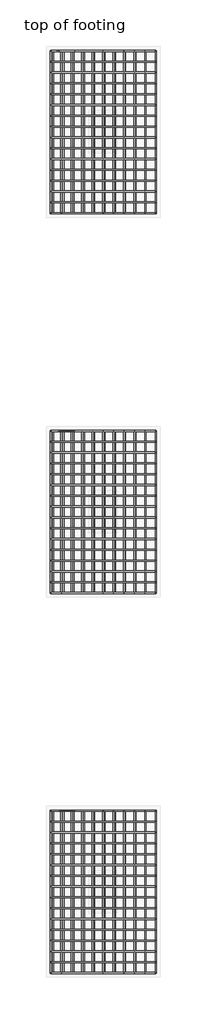
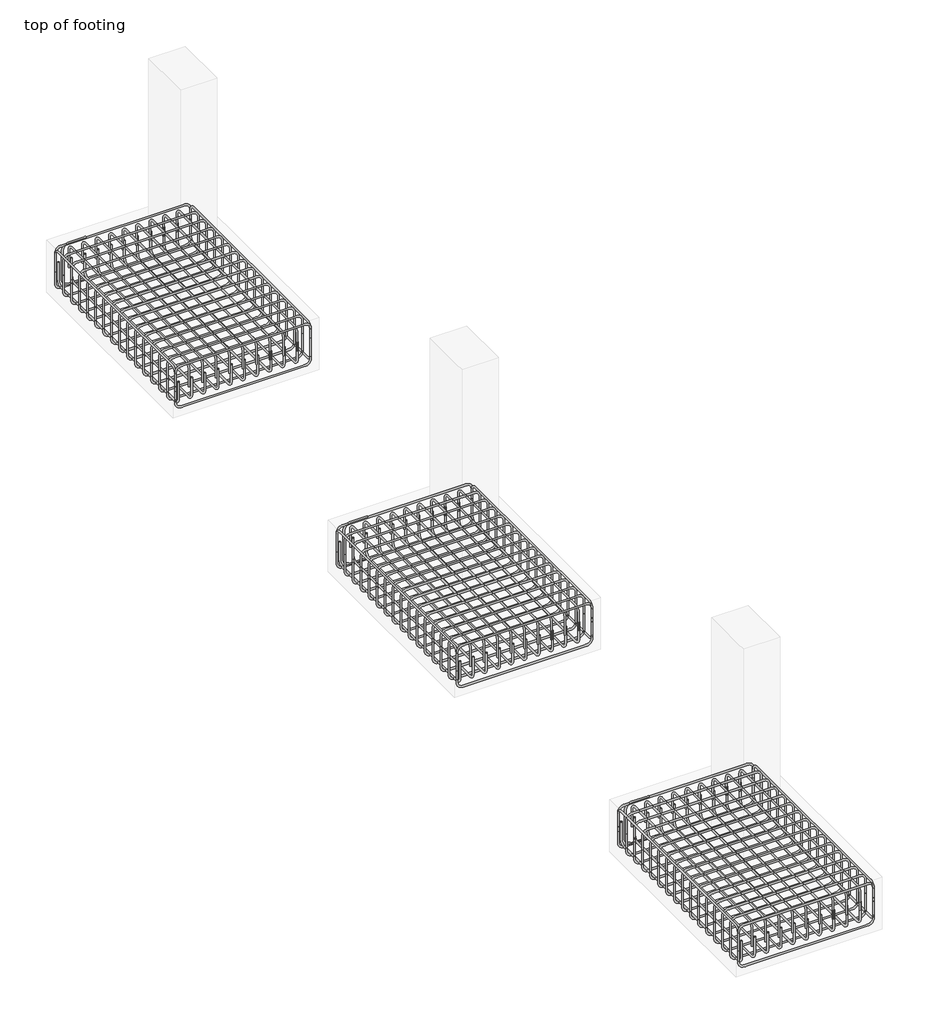
# One storey, part 8 of 8: 15 reinforcing bars.
"""IFC4 building model written with IfcOpenShell, lengths in millimetres."""

from ifc_helpers import new_model, si_unit, point, frame, origin, place, context, project, spatial, polyline, circle_curve, trimmed, segment, composite_curve, source, transform, mapped, element, save
from ifc_brep_helpers import swept_disk

model = new_model("IFC4")

# Units and contexts
model_context = context("Model", 3, world=origin())
ifc_project = project(units=[si_unit("LENGTHUNIT", "METRE", prefix="MILLI")], contexts=[model_context])

# Site, building, storey
site = spatial("IfcSite", under=ifc_project)
building = spatial("IfcBuilding", under=site)
storey = spatial("IfcBuildingStorey", under=building, Name="top of footing", Elevation=-1828.8)

# Reinforcing bars
placement = place(None, origin())
reinforcing_bar_shape = source(origin(), model_context, "Body", "SolidModel", [
    swept_disk(composite_curve([segment(polyline([(3314.5699811, 16682.8075251, -2014.4920065), (3314.5699811, 16682.8075251, -2161.7920065)]), True, "CONTINUOUS"), segment(trimmed(circle_curve(frame((3314.5699811, 16729.1575251, -2161.7920065), z_axis=(1.0, 0.0, 0.0), x_axis=(0.0, -46.349999999998545, 0.0)), 46.35), [point((3314.5699811, 16682.8075251, -2161.7920065))], [point((3314.5699811, 16729.1575251, -2208.1420065))], True, "CARTESIAN"), True, "CONTINUOUS"), segment(polyline([(3314.5699811, 16729.1575251, -2208.1420065), (3314.5699811, 18343.7575251, -2208.1420065)]), True, "CONTINUOUS"), segment(trimmed(circle_curve(frame((3314.5699811, 18343.7575251, -2161.7920065), z_axis=(1.0, 0.0, 0.0), x_axis=(0.0, 0.0, -46.350000000000364)), 46.35), [point((3314.5699811, 18343.7575251, -2208.1420065))], [point((3314.5699811, 18390.1075251, -2161.7920065))], True, "CARTESIAN"), True, "CONTINUOUS"), segment(polyline([(3314.5699811, 18390.1075251, -2161.7920065), (3314.5699811, 18390.1075251, -2014.4920065)]), True, "CONTINUOUS")], self_intersect=False), 6.35),
])
element("IfcReinforcingBar", 1, at=placement, inside=storey, context=model_context, shape_type="MappedRepresentation", body=[
    mapped(reinforcing_bar_shape, transform((0.0, 0.0, 0.0), x_axis=(1.0, 0.0, 0.0), y_axis=(0.0, 1.0, 0.0), z_axis=(0.0, 0.0, 1.0))),
    mapped(reinforcing_bar_shape, transform((-108.3645139, 0.0, 0.0), x_axis=(1.0, 0.0, 0.0), y_axis=(0.0, 1.0, 0.0), z_axis=(0.0, 0.0, 1.0))),
    mapped(reinforcing_bar_shape, transform((-216.7290279, 0.0, 0.0), x_axis=(1.0, 0.0, 0.0), y_axis=(0.0, 1.0, 0.0), z_axis=(0.0, 0.0, 1.0))),
    mapped(reinforcing_bar_shape, transform((-325.0935418, 0.0, 0.0), x_axis=(1.0, 0.0, 0.0), y_axis=(0.0, 1.0, 0.0), z_axis=(0.0, 0.0, 1.0))),
    mapped(reinforcing_bar_shape, transform((-433.4580557, 0.0, 0.0), x_axis=(1.0, 0.0, 0.0), y_axis=(0.0, 1.0, 0.0), z_axis=(0.0, 0.0, 1.0))),
    mapped(reinforcing_bar_shape, transform((-541.8225696, 0.0, 0.0), x_axis=(1.0, 0.0, 0.0), y_axis=(0.0, 1.0, 0.0), z_axis=(0.0, 0.0, 1.0))),
    mapped(reinforcing_bar_shape, transform((-650.1870836, 0.0, 0.0), x_axis=(1.0, 0.0, 0.0), y_axis=(0.0, 1.0, 0.0), z_axis=(0.0, 0.0, 1.0))),
    mapped(reinforcing_bar_shape, transform((-758.5515975, 0.0, 0.0), x_axis=(1.0, 0.0, 0.0), y_axis=(0.0, 1.0, 0.0), z_axis=(0.0, 0.0, 1.0))),
    mapped(reinforcing_bar_shape, transform((-866.9161114, 0.0, 0.0), x_axis=(1.0, 0.0, 0.0), y_axis=(0.0, 1.0, 0.0), z_axis=(0.0, 0.0, 1.0))),
    mapped(reinforcing_bar_shape, transform((-975.2806253, 0.0, 0.0), x_axis=(1.0, 0.0, 0.0), y_axis=(0.0, 1.0, 0.0), z_axis=(0.0, 0.0, 1.0))),
    mapped(reinforcing_bar_shape, transform((-1083.6451393, 0.0, 0.0), x_axis=(1.0, 0.0, 0.0), y_axis=(0.0, 1.0, 0.0), z_axis=(0.0, 0.0, 1.0))),
])
reinforcing_bar_2_shape = source(origin(), model_context, "Body", "SolidModel", [
    swept_disk(composite_curve([segment(polyline([(2207.2699811, 16682.8075251, -2085.8010212), (2207.2699811, 16682.8075251, -1938.5010212)]), True, "CONTINUOUS"), segment(trimmed(circle_curve(frame((2207.2699811, 16729.1575251, -1938.5010212), z_axis=(-1.0, 0.0, 0.0), x_axis=(0.0, -46.349999999998545, 0.0)), 46.35), [point((2207.2699811, 16682.8075251, -1938.5010212))], [point((2207.2699811, 16729.1575251, -1892.1510212))], True, "CARTESIAN"), True, "CONTINUOUS"), segment(polyline([(2207.2699811, 16729.1575251, -1892.1510212), (2207.2699811, 18343.7575251, -1892.1510212)]), True, "CONTINUOUS"), segment(trimmed(circle_curve(frame((2207.2699811, 18343.7575251, -1938.5010212), z_axis=(-1.0, 0.0, 0.0), x_axis=(0.0, 0.0, 46.34999999999991)), 46.35), [point((2207.2699811, 18343.7575251, -1892.1510212))], [point((2207.2699811, 18390.1075251, -1938.5010212))], True, "CARTESIAN"), True, "CONTINUOUS"), segment(polyline([(2207.2699811, 18390.1075251, -1938.5010212), (2207.2699811, 18390.1075251, -2085.8010212)]), True, "CONTINUOUS")], self_intersect=False), 6.35),
])
element("IfcReinforcingBar", 2, at=placement, inside=storey, context=model_context, shape_type="MappedRepresentation", body=[
    mapped(reinforcing_bar_2_shape, transform((0.0, 0.0, 0.0), x_axis=(1.0, 0.0, 0.0), y_axis=(0.0, 1.0, 0.0), z_axis=(0.0, 0.0, 1.0))),
    mapped(reinforcing_bar_2_shape, transform((110.73, 0.0, 0.0), x_axis=(1.0, 0.0, 0.0), y_axis=(0.0, 1.0, 0.0), z_axis=(0.0, 0.0, 1.0))),
    mapped(reinforcing_bar_2_shape, transform((221.46, 0.0, 0.0), x_axis=(1.0, 0.0, 0.0), y_axis=(0.0, 1.0, 0.0), z_axis=(0.0, 0.0, 1.0))),
    mapped(reinforcing_bar_2_shape, transform((332.19, 0.0, 0.0), x_axis=(1.0, 0.0, 0.0), y_axis=(0.0, 1.0, 0.0), z_axis=(0.0, 0.0, 1.0))),
    mapped(reinforcing_bar_2_shape, transform((442.92, 0.0, 0.0), x_axis=(1.0, 0.0, 0.0), y_axis=(0.0, 1.0, 0.0), z_axis=(0.0, 0.0, 1.0))),
    mapped(reinforcing_bar_2_shape, transform((553.65, 0.0, 0.0), x_axis=(1.0, 0.0, 0.0), y_axis=(0.0, 1.0, 0.0), z_axis=(0.0, 0.0, 1.0))),
    mapped(reinforcing_bar_2_shape, transform((664.38, 0.0, 0.0), x_axis=(1.0, 0.0, 0.0), y_axis=(0.0, 1.0, 0.0), z_axis=(0.0, 0.0, 1.0))),
    mapped(reinforcing_bar_2_shape, transform((775.11, 0.0, 0.0), x_axis=(1.0, 0.0, 0.0), y_axis=(0.0, 1.0, 0.0), z_axis=(0.0, 0.0, 1.0))),
    mapped(reinforcing_bar_2_shape, transform((885.84, 0.0, 0.0), x_axis=(1.0, 0.0, 0.0), y_axis=(0.0, 1.0, 0.0), z_axis=(0.0, 0.0, 1.0))),
    mapped(reinforcing_bar_2_shape, transform((996.57, 0.0, 0.0), x_axis=(1.0, 0.0, 0.0), y_axis=(0.0, 1.0, 0.0), z_axis=(0.0, 0.0, 1.0))),
    mapped(reinforcing_bar_2_shape, transform((1107.3, 0.0, 0.0), x_axis=(1.0, 0.0, 0.0), y_axis=(0.0, 1.0, 0.0), z_axis=(0.0, 0.0, 1.0))),
])
element("IfcReinforcingBar", 3, at=placement, inside=storey, context=model_context, shape_type="SolidModel", body=[
    swept_disk(composite_curve([segment(polyline([(2456.9690895, 18390.1075251, -2232.45), (2309.6690895, 18390.1075251, -2232.45)]), True, "CONTINUOUS"), segment(trimmed(circle_curve(frame((2309.6690895, 18390.1075251, -2186.1), z_axis=(0.0, 1.0, 0.0), x_axis=(0.0, 0.0, -46.34999999999991)), 46.35), [point((2309.6690895, 18390.1075251, -2232.45))], [point((2263.3190895, 18390.1075251, -2186.1))], True, "CARTESIAN"), True, "CONTINUOUS"), segment(polyline([(2263.3190895, 18390.1075251, -2186.1), (2263.3190895, 18390.1075251, -1921.5)]), True, "CONTINUOUS"), segment(trimmed(circle_curve(frame((2309.6690895, 18390.1075251, -1921.5), z_axis=(0.0, 1.0, 0.0), x_axis=(-46.350000000000364, 0.0, 0.0)), 46.35), [point((2263.3190895, 18390.1075251, -1921.5))], [point((2309.6690895, 18390.1075251, -1875.15))], True, "CARTESIAN"), True, "CONTINUOUS"), segment(polyline([(2309.6690895, 18390.1075251, -1875.15), (2456.9690895, 18390.1075251, -1875.15)]), True, "CONTINUOUS")], self_intersect=False), 6.35),
])
reinforcing_bar_3_shape = source(origin(), model_context, "Body", "SolidModel", [
    swept_disk(composite_curve([segment(polyline([(3314.5699811, 18390.1075251, -2044.8290141), (3314.5699811, 18390.1075251, -2192.1290141)]), True, "CONTINUOUS"), segment(trimmed(circle_curve(frame((3268.2199811, 18390.1075251, -2192.1290141), z_axis=(0.0, 1.0, 0.0), x_axis=(46.34999999999991, 0.0, 0.0)), 46.35), [point((3314.5699811, 18390.1075251, -2192.1290141))], [point((3268.2199811, 18390.1075251, -2238.4790141))], True, "CARTESIAN"), True, "CONTINUOUS"), segment(polyline([(3268.2199811, 18390.1075251, -2238.4790141), (2253.6199811, 18390.1075251, -2238.4790141)]), True, "CONTINUOUS"), segment(trimmed(circle_curve(frame((2253.6199811, 18390.1075251, -2192.1290141), z_axis=(0.0, 1.0, 0.0), x_axis=(0.0, 0.0, -46.34999999999991)), 46.35), [point((2253.6199811, 18390.1075251, -2238.4790141))], [point((2207.2699811, 18390.1075251, -2192.1290141))], True, "CARTESIAN"), True, "CONTINUOUS"), segment(polyline([(2207.2699811, 18390.1075251, -2192.1290141), (2207.2699811, 18390.1075251, -2044.8290141)]), True, "CONTINUOUS")], self_intersect=False), 6.35),
])
element("IfcReinforcingBar", 4, at=placement, inside=storey, context=model_context, shape_type="MappedRepresentation", body=[
    mapped(reinforcing_bar_3_shape, transform((0.0, 0.0, 0.0), x_axis=(1.0, 0.0, 0.0), y_axis=(0.0, 1.0, 0.0), z_axis=(0.0, 0.0, 1.0))),
    mapped(reinforcing_bar_3_shape, transform((0.0, -113.82, 0.0), x_axis=(1.0, 0.0, 0.0), y_axis=(0.0, 1.0, 0.0), z_axis=(0.0, 0.0, 1.0))),
    mapped(reinforcing_bar_3_shape, transform((0.0, -227.64, 0.0), x_axis=(1.0, 0.0, 0.0), y_axis=(0.0, 1.0, 0.0), z_axis=(0.0, 0.0, 1.0))),
    mapped(reinforcing_bar_3_shape, transform((0.0, -341.46, 0.0), x_axis=(1.0, 0.0, 0.0), y_axis=(0.0, 1.0, 0.0), z_axis=(0.0, 0.0, 1.0))),
    mapped(reinforcing_bar_3_shape, transform((0.0, -455.28, 0.0), x_axis=(1.0, 0.0, 0.0), y_axis=(0.0, 1.0, 0.0), z_axis=(0.0, 0.0, 1.0))),
    mapped(reinforcing_bar_3_shape, transform((0.0, -569.1, 0.0), x_axis=(1.0, 0.0, 0.0), y_axis=(0.0, 1.0, 0.0), z_axis=(0.0, 0.0, 1.0))),
    mapped(reinforcing_bar_3_shape, transform((0.0, -682.92, 0.0), x_axis=(1.0, 0.0, 0.0), y_axis=(0.0, 1.0, 0.0), z_axis=(0.0, 0.0, 1.0))),
    mapped(reinforcing_bar_3_shape, transform((0.0, -796.74, 0.0), x_axis=(1.0, 0.0, 0.0), y_axis=(0.0, 1.0, 0.0), z_axis=(0.0, 0.0, 1.0))),
    mapped(reinforcing_bar_3_shape, transform((0.0, -910.56, 0.0), x_axis=(1.0, 0.0, 0.0), y_axis=(0.0, 1.0, 0.0), z_axis=(0.0, 0.0, 1.0))),
    mapped(reinforcing_bar_3_shape, transform((0.0, -1024.38, 0.0), x_axis=(1.0, 0.0, 0.0), y_axis=(0.0, 1.0, 0.0), z_axis=(0.0, 0.0, 1.0))),
    mapped(reinforcing_bar_3_shape, transform((0.0, -1138.2, 0.0), x_axis=(1.0, 0.0, 0.0), y_axis=(0.0, 1.0, 0.0), z_axis=(0.0, 0.0, 1.0))),
    mapped(reinforcing_bar_3_shape, transform((0.0, -1252.02, 0.0), x_axis=(1.0, 0.0, 0.0), y_axis=(0.0, 1.0, 0.0), z_axis=(0.0, 0.0, 1.0))),
    mapped(reinforcing_bar_3_shape, transform((0.0, -1365.84, 0.0), x_axis=(1.0, 0.0, 0.0), y_axis=(0.0, 1.0, 0.0), z_axis=(0.0, 0.0, 1.0))),
    mapped(reinforcing_bar_3_shape, transform((0.0, -1479.66, 0.0), x_axis=(1.0, 0.0, 0.0), y_axis=(0.0, 1.0, 0.0), z_axis=(0.0, 0.0, 1.0))),
    mapped(reinforcing_bar_3_shape, transform((0.0, -1593.48, 0.0), x_axis=(1.0, 0.0, 0.0), y_axis=(0.0, 1.0, 0.0), z_axis=(0.0, 0.0, 1.0))),
    mapped(reinforcing_bar_3_shape, transform((0.0, -1707.3, 0.0), x_axis=(1.0, 0.0, 0.0), y_axis=(0.0, 1.0, 0.0), z_axis=(0.0, 0.0, 1.0))),
])
reinforcing_bar_4_shape = source(origin(), model_context, "Body", "SolidModel", [
    swept_disk(composite_curve([segment(polyline([(2207.2699811, 18390.1075251, -2075.0801535), (2207.2699811, 18390.1075251, -1927.7801535)]), True, "CONTINUOUS"), segment(trimmed(circle_curve(frame((2253.6199811, 18390.1075251, -1927.7801535), z_axis=(0.0, 1.0, 0.0), x_axis=(-46.34999999999991, 0.0, 0.0)), 46.35), [point((2207.2699811, 18390.1075251, -1927.7801535))], [point((2253.6199811, 18390.1075251, -1881.4301535))], True, "CARTESIAN"), True, "CONTINUOUS"), segment(polyline([(2253.6199811, 18390.1075251, -1881.4301535), (3268.2199811, 18390.1075251, -1881.4301535)]), True, "CONTINUOUS"), segment(trimmed(circle_curve(frame((3268.2199811, 18390.1075251, -1927.7801535), z_axis=(0.0, 1.0, 0.0), x_axis=(0.0, 0.0, 46.350000000000136)), 46.35), [point((3268.2199811, 18390.1075251, -1881.4301535))], [point((3314.5699811, 18390.1075251, -1927.7801535))], True, "CARTESIAN"), True, "CONTINUOUS"), segment(polyline([(3314.5699811, 18390.1075251, -1927.7801535), (3314.5699811, 18390.1075251, -2075.0801535)]), True, "CONTINUOUS")], self_intersect=False), 6.35),
])
element("IfcReinforcingBar", 5, at=placement, inside=storey, context=model_context, shape_type="MappedRepresentation", body=[
    mapped(reinforcing_bar_4_shape, transform((0.0, 0.0, 0.0), x_axis=(1.0, 0.0, 0.0), y_axis=(0.0, 1.0, 0.0), z_axis=(0.0, 0.0, 1.0))),
    mapped(reinforcing_bar_4_shape, transform((0.0, -113.82, 0.0), x_axis=(1.0, 0.0, 0.0), y_axis=(0.0, 1.0, 0.0), z_axis=(0.0, 0.0, 1.0))),
    mapped(reinforcing_bar_4_shape, transform((0.0, -227.64, 0.0), x_axis=(1.0, 0.0, 0.0), y_axis=(0.0, 1.0, 0.0), z_axis=(0.0, 0.0, 1.0))),
    mapped(reinforcing_bar_4_shape, transform((0.0, -341.46, 0.0), x_axis=(1.0, 0.0, 0.0), y_axis=(0.0, 1.0, 0.0), z_axis=(0.0, 0.0, 1.0))),
    mapped(reinforcing_bar_4_shape, transform((0.0, -455.28, 0.0), x_axis=(1.0, 0.0, 0.0), y_axis=(0.0, 1.0, 0.0), z_axis=(0.0, 0.0, 1.0))),
    mapped(reinforcing_bar_4_shape, transform((0.0, -569.1, 0.0), x_axis=(1.0, 0.0, 0.0), y_axis=(0.0, 1.0, 0.0), z_axis=(0.0, 0.0, 1.0))),
    mapped(reinforcing_bar_4_shape, transform((0.0, -682.92, 0.0), x_axis=(1.0, 0.0, 0.0), y_axis=(0.0, 1.0, 0.0), z_axis=(0.0, 0.0, 1.0))),
    mapped(reinforcing_bar_4_shape, transform((0.0, -796.74, 0.0), x_axis=(1.0, 0.0, 0.0), y_axis=(0.0, 1.0, 0.0), z_axis=(0.0, 0.0, 1.0))),
    mapped(reinforcing_bar_4_shape, transform((0.0, -910.56, 0.0), x_axis=(1.0, 0.0, 0.0), y_axis=(0.0, 1.0, 0.0), z_axis=(0.0, 0.0, 1.0))),
    mapped(reinforcing_bar_4_shape, transform((0.0, -1024.38, 0.0), x_axis=(1.0, 0.0, 0.0), y_axis=(0.0, 1.0, 0.0), z_axis=(0.0, 0.0, 1.0))),
    mapped(reinforcing_bar_4_shape, transform((0.0, -1138.2, 0.0), x_axis=(1.0, 0.0, 0.0), y_axis=(0.0, 1.0, 0.0), z_axis=(0.0, 0.0, 1.0))),
    mapped(reinforcing_bar_4_shape, transform((0.0, -1252.02, 0.0), x_axis=(1.0, 0.0, 0.0), y_axis=(0.0, 1.0, 0.0), z_axis=(0.0, 0.0, 1.0))),
    mapped(reinforcing_bar_4_shape, transform((0.0, -1365.84, 0.0), x_axis=(1.0, 0.0, 0.0), y_axis=(0.0, 1.0, 0.0), z_axis=(0.0, 0.0, 1.0))),
    mapped(reinforcing_bar_4_shape, transform((0.0, -1479.66, 0.0), x_axis=(1.0, 0.0, 0.0), y_axis=(0.0, 1.0, 0.0), z_axis=(0.0, 0.0, 1.0))),
    mapped(reinforcing_bar_4_shape, transform((0.0, -1593.48, 0.0), x_axis=(1.0, 0.0, 0.0), y_axis=(0.0, 1.0, 0.0), z_axis=(0.0, 0.0, 1.0))),
    mapped(reinforcing_bar_4_shape, transform((0.0, -1707.3, 0.0), x_axis=(1.0, 0.0, 0.0), y_axis=(0.0, 1.0, 0.0), z_axis=(0.0, 0.0, 1.0))),
])
reinforcing_bar_5_shape = source(origin(), model_context, "Body", "SolidModel", [
    swept_disk(composite_curve([segment(polyline([(3314.5699811, 12682.8075251, -2014.4920065), (3314.5699811, 12682.8075251, -2161.7920065)]), True, "CONTINUOUS"), segment(trimmed(circle_curve(frame((3314.5699811, 12729.1575251, -2161.7920065), z_axis=(1.0, 0.0, 0.0), x_axis=(0.0, -46.350000000000364, 0.0)), 46.35), [point((3314.5699811, 12682.8075251, -2161.7920065))], [point((3314.5699811, 12729.1575251, -2208.1420065))], True, "CARTESIAN"), True, "CONTINUOUS"), segment(polyline([(3314.5699811, 12729.1575251, -2208.1420065), (3314.5699811, 14343.7575251, -2208.1420065)]), True, "CONTINUOUS"), segment(trimmed(circle_curve(frame((3314.5699811, 14343.7575251, -2161.7920065), z_axis=(1.0, 0.0, 0.0), x_axis=(0.0, 0.0, -46.350000000000364)), 46.35), [point((3314.5699811, 14343.7575251, -2208.1420065))], [point((3314.5699811, 14390.1075251, -2161.7920065))], True, "CARTESIAN"), True, "CONTINUOUS"), segment(polyline([(3314.5699811, 14390.1075251, -2161.7920065), (3314.5699811, 14390.1075251, -2014.4920065)]), True, "CONTINUOUS")], self_intersect=False), 6.35),
])
element("IfcReinforcingBar", 6, at=placement, inside=storey, context=model_context, shape_type="MappedRepresentation", body=[
    mapped(reinforcing_bar_5_shape, transform((0.0, 0.0, 0.0), x_axis=(1.0, 0.0, 0.0), y_axis=(0.0, 1.0, 0.0), z_axis=(0.0, 0.0, 1.0))),
    mapped(reinforcing_bar_5_shape, transform((-108.3645139, 0.0, 0.0), x_axis=(1.0, 0.0, 0.0), y_axis=(0.0, 1.0, 0.0), z_axis=(0.0, 0.0, 1.0))),
    mapped(reinforcing_bar_5_shape, transform((-216.7290279, 0.0, 0.0), x_axis=(1.0, 0.0, 0.0), y_axis=(0.0, 1.0, 0.0), z_axis=(0.0, 0.0, 1.0))),
    mapped(reinforcing_bar_5_shape, transform((-325.0935418, 0.0, 0.0), x_axis=(1.0, 0.0, 0.0), y_axis=(0.0, 1.0, 0.0), z_axis=(0.0, 0.0, 1.0))),
    mapped(reinforcing_bar_5_shape, transform((-433.4580557, 0.0, 0.0), x_axis=(1.0, 0.0, 0.0), y_axis=(0.0, 1.0, 0.0), z_axis=(0.0, 0.0, 1.0))),
    mapped(reinforcing_bar_5_shape, transform((-541.8225696, 0.0, 0.0), x_axis=(1.0, 0.0, 0.0), y_axis=(0.0, 1.0, 0.0), z_axis=(0.0, 0.0, 1.0))),
    mapped(reinforcing_bar_5_shape, transform((-650.1870836, 0.0, 0.0), x_axis=(1.0, 0.0, 0.0), y_axis=(0.0, 1.0, 0.0), z_axis=(0.0, 0.0, 1.0))),
    mapped(reinforcing_bar_5_shape, transform((-758.5515975, 0.0, 0.0), x_axis=(1.0, 0.0, 0.0), y_axis=(0.0, 1.0, 0.0), z_axis=(0.0, 0.0, 1.0))),
    mapped(reinforcing_bar_5_shape, transform((-866.9161114, 0.0, 0.0), x_axis=(1.0, 0.0, 0.0), y_axis=(0.0, 1.0, 0.0), z_axis=(0.0, 0.0, 1.0))),
    mapped(reinforcing_bar_5_shape, transform((-975.2806253, 0.0, 0.0), x_axis=(1.0, 0.0, 0.0), y_axis=(0.0, 1.0, 0.0), z_axis=(0.0, 0.0, 1.0))),
    mapped(reinforcing_bar_5_shape, transform((-1083.6451393, 0.0, 0.0), x_axis=(1.0, 0.0, 0.0), y_axis=(0.0, 1.0, 0.0), z_axis=(0.0, 0.0, 1.0))),
])
reinforcing_bar_6_shape = source(origin(), model_context, "Body", "SolidModel", [
    swept_disk(composite_curve([segment(polyline([(2207.2699811, 12682.8075251, -2085.8010212), (2207.2699811, 12682.8075251, -1938.5010212)]), True, "CONTINUOUS"), segment(trimmed(circle_curve(frame((2207.2699811, 12729.1575251, -1938.5010212), z_axis=(-1.0, 0.0, 0.0), x_axis=(0.0, -46.350000000000364, 0.0)), 46.35), [point((2207.2699811, 12682.8075251, -1938.5010212))], [point((2207.2699811, 12729.1575251, -1892.1510212))], True, "CARTESIAN"), True, "CONTINUOUS"), segment(polyline([(2207.2699811, 12729.1575251, -1892.1510212), (2207.2699811, 14343.7575251, -1892.1510212)]), True, "CONTINUOUS"), segment(trimmed(circle_curve(frame((2207.2699811, 14343.7575251, -1938.5010212), z_axis=(-1.0, 0.0, 0.0), x_axis=(0.0, 0.0, 46.34999999999991)), 46.35), [point((2207.2699811, 14343.7575251, -1892.1510212))], [point((2207.2699811, 14390.1075251, -1938.5010212))], True, "CARTESIAN"), True, "CONTINUOUS"), segment(polyline([(2207.2699811, 14390.1075251, -1938.5010212), (2207.2699811, 14390.1075251, -2085.8010212)]), True, "CONTINUOUS")], self_intersect=False), 6.35),
])
element("IfcReinforcingBar", 7, at=placement, inside=storey, context=model_context, shape_type="MappedRepresentation", body=[
    mapped(reinforcing_bar_6_shape, transform((0.0, 0.0, 0.0), x_axis=(1.0, 0.0, 0.0), y_axis=(0.0, 1.0, 0.0), z_axis=(0.0, 0.0, 1.0))),
    mapped(reinforcing_bar_6_shape, transform((110.73, 0.0, 0.0), x_axis=(1.0, 0.0, 0.0), y_axis=(0.0, 1.0, 0.0), z_axis=(0.0, 0.0, 1.0))),
    mapped(reinforcing_bar_6_shape, transform((221.46, 0.0, 0.0), x_axis=(1.0, 0.0, 0.0), y_axis=(0.0, 1.0, 0.0), z_axis=(0.0, 0.0, 1.0))),
    mapped(reinforcing_bar_6_shape, transform((332.19, 0.0, 0.0), x_axis=(1.0, 0.0, 0.0), y_axis=(0.0, 1.0, 0.0), z_axis=(0.0, 0.0, 1.0))),
    mapped(reinforcing_bar_6_shape, transform((442.92, 0.0, 0.0), x_axis=(1.0, 0.0, 0.0), y_axis=(0.0, 1.0, 0.0), z_axis=(0.0, 0.0, 1.0))),
    mapped(reinforcing_bar_6_shape, transform((553.65, 0.0, 0.0), x_axis=(1.0, 0.0, 0.0), y_axis=(0.0, 1.0, 0.0), z_axis=(0.0, 0.0, 1.0))),
    mapped(reinforcing_bar_6_shape, transform((664.38, 0.0, 0.0), x_axis=(1.0, 0.0, 0.0), y_axis=(0.0, 1.0, 0.0), z_axis=(0.0, 0.0, 1.0))),
    mapped(reinforcing_bar_6_shape, transform((775.11, 0.0, 0.0), x_axis=(1.0, 0.0, 0.0), y_axis=(0.0, 1.0, 0.0), z_axis=(0.0, 0.0, 1.0))),
    mapped(reinforcing_bar_6_shape, transform((885.84, 0.0, 0.0), x_axis=(1.0, 0.0, 0.0), y_axis=(0.0, 1.0, 0.0), z_axis=(0.0, 0.0, 1.0))),
    mapped(reinforcing_bar_6_shape, transform((996.57, 0.0, 0.0), x_axis=(1.0, 0.0, 0.0), y_axis=(0.0, 1.0, 0.0), z_axis=(0.0, 0.0, 1.0))),
    mapped(reinforcing_bar_6_shape, transform((1107.3, 0.0, 0.0), x_axis=(1.0, 0.0, 0.0), y_axis=(0.0, 1.0, 0.0), z_axis=(0.0, 0.0, 1.0))),
])
element("IfcReinforcingBar", 8, at=placement, inside=storey, context=model_context, shape_type="SolidModel", body=[
    swept_disk(composite_curve([segment(polyline([(2456.9690895, 14390.1075251, -2232.45), (2309.6690895, 14390.1075251, -2232.45)]), True, "CONTINUOUS"), segment(trimmed(circle_curve(frame((2309.6690895, 14390.1075251, -2186.1), z_axis=(0.0, 1.0, 0.0), x_axis=(0.0, 0.0, -46.34999999999991)), 46.35), [point((2309.6690895, 14390.1075251, -2232.45))], [point((2263.3190895, 14390.1075251, -2186.1))], True, "CARTESIAN"), True, "CONTINUOUS"), segment(polyline([(2263.3190895, 14390.1075251, -2186.1), (2263.3190895, 14390.1075251, -1921.5)]), True, "CONTINUOUS"), segment(trimmed(circle_curve(frame((2309.6690895, 14390.1075251, -1921.5), z_axis=(0.0, 1.0, 0.0), x_axis=(-46.350000000000364, 0.0, 0.0)), 46.35), [point((2263.3190895, 14390.1075251, -1921.5))], [point((2309.6690895, 14390.1075251, -1875.15))], True, "CARTESIAN"), True, "CONTINUOUS"), segment(polyline([(2309.6690895, 14390.1075251, -1875.15), (2456.9690895, 14390.1075251, -1875.15)]), True, "CONTINUOUS")], self_intersect=False), 6.35),
])
reinforcing_bar_7_shape = source(origin(), model_context, "Body", "SolidModel", [
    swept_disk(composite_curve([segment(polyline([(3314.5699811, 14390.1075251, -2044.8290141), (3314.5699811, 14390.1075251, -2192.1290141)]), True, "CONTINUOUS"), segment(trimmed(circle_curve(frame((3268.2199811, 14390.1075251, -2192.1290141), z_axis=(0.0, 1.0, 0.0), x_axis=(46.34999999999991, 0.0, 0.0)), 46.35), [point((3314.5699811, 14390.1075251, -2192.1290141))], [point((3268.2199811, 14390.1075251, -2238.4790141))], True, "CARTESIAN"), True, "CONTINUOUS"), segment(polyline([(3268.2199811, 14390.1075251, -2238.4790141), (2253.6199811, 14390.1075251, -2238.4790141)]), True, "CONTINUOUS"), segment(trimmed(circle_curve(frame((2253.6199811, 14390.1075251, -2192.1290141), z_axis=(0.0, 1.0, 0.0), x_axis=(0.0, 0.0, -46.34999999999991)), 46.35), [point((2253.6199811, 14390.1075251, -2238.4790141))], [point((2207.2699811, 14390.1075251, -2192.1290141))], True, "CARTESIAN"), True, "CONTINUOUS"), segment(polyline([(2207.2699811, 14390.1075251, -2192.1290141), (2207.2699811, 14390.1075251, -2044.8290141)]), True, "CONTINUOUS")], self_intersect=False), 6.35),
])
element("IfcReinforcingBar", 9, at=placement, inside=storey, context=model_context, shape_type="MappedRepresentation", body=[
    mapped(reinforcing_bar_7_shape, transform((0.0, 0.0, 0.0), x_axis=(1.0, 0.0, 0.0), y_axis=(0.0, 1.0, 0.0), z_axis=(0.0, 0.0, 1.0))),
    mapped(reinforcing_bar_7_shape, transform((0.0, -113.82, 0.0), x_axis=(1.0, 0.0, 0.0), y_axis=(0.0, 1.0, 0.0), z_axis=(0.0, 0.0, 1.0))),
    mapped(reinforcing_bar_7_shape, transform((0.0, -227.64, 0.0), x_axis=(1.0, 0.0, 0.0), y_axis=(0.0, 1.0, 0.0), z_axis=(0.0, 0.0, 1.0))),
    mapped(reinforcing_bar_7_shape, transform((0.0, -341.46, 0.0), x_axis=(1.0, 0.0, 0.0), y_axis=(0.0, 1.0, 0.0), z_axis=(0.0, 0.0, 1.0))),
    mapped(reinforcing_bar_7_shape, transform((0.0, -455.28, 0.0), x_axis=(1.0, 0.0, 0.0), y_axis=(0.0, 1.0, 0.0), z_axis=(0.0, 0.0, 1.0))),
    mapped(reinforcing_bar_7_shape, transform((0.0, -569.1, 0.0), x_axis=(1.0, 0.0, 0.0), y_axis=(0.0, 1.0, 0.0), z_axis=(0.0, 0.0, 1.0))),
    mapped(reinforcing_bar_7_shape, transform((0.0, -682.92, 0.0), x_axis=(1.0, 0.0, 0.0), y_axis=(0.0, 1.0, 0.0), z_axis=(0.0, 0.0, 1.0))),
    mapped(reinforcing_bar_7_shape, transform((0.0, -796.74, 0.0), x_axis=(1.0, 0.0, 0.0), y_axis=(0.0, 1.0, 0.0), z_axis=(0.0, 0.0, 1.0))),
    mapped(reinforcing_bar_7_shape, transform((0.0, -910.56, 0.0), x_axis=(1.0, 0.0, 0.0), y_axis=(0.0, 1.0, 0.0), z_axis=(0.0, 0.0, 1.0))),
    mapped(reinforcing_bar_7_shape, transform((0.0, -1024.38, 0.0), x_axis=(1.0, 0.0, 0.0), y_axis=(0.0, 1.0, 0.0), z_axis=(0.0, 0.0, 1.0))),
    mapped(reinforcing_bar_7_shape, transform((0.0, -1138.2, 0.0), x_axis=(1.0, 0.0, 0.0), y_axis=(0.0, 1.0, 0.0), z_axis=(0.0, 0.0, 1.0))),
    mapped(reinforcing_bar_7_shape, transform((0.0, -1252.02, 0.0), x_axis=(1.0, 0.0, 0.0), y_axis=(0.0, 1.0, 0.0), z_axis=(0.0, 0.0, 1.0))),
    mapped(reinforcing_bar_7_shape, transform((0.0, -1365.84, 0.0), x_axis=(1.0, 0.0, 0.0), y_axis=(0.0, 1.0, 0.0), z_axis=(0.0, 0.0, 1.0))),
    mapped(reinforcing_bar_7_shape, transform((0.0, -1479.66, 0.0), x_axis=(1.0, 0.0, 0.0), y_axis=(0.0, 1.0, 0.0), z_axis=(0.0, 0.0, 1.0))),
    mapped(reinforcing_bar_7_shape, transform((0.0, -1593.48, 0.0), x_axis=(1.0, 0.0, 0.0), y_axis=(0.0, 1.0, 0.0), z_axis=(0.0, 0.0, 1.0))),
    mapped(reinforcing_bar_7_shape, transform((0.0, -1707.3, 0.0), x_axis=(1.0, 0.0, 0.0), y_axis=(0.0, 1.0, 0.0), z_axis=(0.0, 0.0, 1.0))),
])
reinforcing_bar_8_shape = source(origin(), model_context, "Body", "SolidModel", [
    swept_disk(composite_curve([segment(polyline([(2207.2699811, 14390.1075251, -2075.0801535), (2207.2699811, 14390.1075251, -1927.7801535)]), True, "CONTINUOUS"), segment(trimmed(circle_curve(frame((2253.6199811, 14390.1075251, -1927.7801535), z_axis=(0.0, 1.0, 0.0), x_axis=(-46.34999999999991, 0.0, 0.0)), 46.35), [point((2207.2699811, 14390.1075251, -1927.7801535))], [point((2253.6199811, 14390.1075251, -1881.4301535))], True, "CARTESIAN"), True, "CONTINUOUS"), segment(polyline([(2253.6199811, 14390.1075251, -1881.4301535), (3268.2199811, 14390.1075251, -1881.4301535)]), True, "CONTINUOUS"), segment(trimmed(circle_curve(frame((3268.2199811, 14390.1075251, -1927.7801535), z_axis=(0.0, 1.0, 0.0), x_axis=(0.0, 0.0, 46.350000000000136)), 46.35), [point((3268.2199811, 14390.1075251, -1881.4301535))], [point((3314.5699811, 14390.1075251, -1927.7801535))], True, "CARTESIAN"), True, "CONTINUOUS"), segment(polyline([(3314.5699811, 14390.1075251, -1927.7801535), (3314.5699811, 14390.1075251, -2075.0801535)]), True, "CONTINUOUS")], self_intersect=False), 6.35),
])
element("IfcReinforcingBar", 10, at=placement, inside=storey, context=model_context, shape_type="MappedRepresentation", body=[
    mapped(reinforcing_bar_8_shape, transform((0.0, 0.0, 0.0), x_axis=(1.0, 0.0, 0.0), y_axis=(0.0, 1.0, 0.0), z_axis=(0.0, 0.0, 1.0))),
    mapped(reinforcing_bar_8_shape, transform((0.0, -113.82, 0.0), x_axis=(1.0, 0.0, 0.0), y_axis=(0.0, 1.0, 0.0), z_axis=(0.0, 0.0, 1.0))),
    mapped(reinforcing_bar_8_shape, transform((0.0, -227.64, 0.0), x_axis=(1.0, 0.0, 0.0), y_axis=(0.0, 1.0, 0.0), z_axis=(0.0, 0.0, 1.0))),
    mapped(reinforcing_bar_8_shape, transform((0.0, -341.46, 0.0), x_axis=(1.0, 0.0, 0.0), y_axis=(0.0, 1.0, 0.0), z_axis=(0.0, 0.0, 1.0))),
    mapped(reinforcing_bar_8_shape, transform((0.0, -455.28, 0.0), x_axis=(1.0, 0.0, 0.0), y_axis=(0.0, 1.0, 0.0), z_axis=(0.0, 0.0, 1.0))),
    mapped(reinforcing_bar_8_shape, transform((0.0, -569.1, 0.0), x_axis=(1.0, 0.0, 0.0), y_axis=(0.0, 1.0, 0.0), z_axis=(0.0, 0.0, 1.0))),
    mapped(reinforcing_bar_8_shape, transform((0.0, -682.92, 0.0), x_axis=(1.0, 0.0, 0.0), y_axis=(0.0, 1.0, 0.0), z_axis=(0.0, 0.0, 1.0))),
    mapped(reinforcing_bar_8_shape, transform((0.0, -796.74, 0.0), x_axis=(1.0, 0.0, 0.0), y_axis=(0.0, 1.0, 0.0), z_axis=(0.0, 0.0, 1.0))),
    mapped(reinforcing_bar_8_shape, transform((0.0, -910.56, 0.0), x_axis=(1.0, 0.0, 0.0), y_axis=(0.0, 1.0, 0.0), z_axis=(0.0, 0.0, 1.0))),
    mapped(reinforcing_bar_8_shape, transform((0.0, -1024.38, 0.0), x_axis=(1.0, 0.0, 0.0), y_axis=(0.0, 1.0, 0.0), z_axis=(0.0, 0.0, 1.0))),
    mapped(reinforcing_bar_8_shape, transform((0.0, -1138.2, 0.0), x_axis=(1.0, 0.0, 0.0), y_axis=(0.0, 1.0, 0.0), z_axis=(0.0, 0.0, 1.0))),
    mapped(reinforcing_bar_8_shape, transform((0.0, -1252.02, 0.0), x_axis=(1.0, 0.0, 0.0), y_axis=(0.0, 1.0, 0.0), z_axis=(0.0, 0.0, 1.0))),
    mapped(reinforcing_bar_8_shape, transform((0.0, -1365.84, 0.0), x_axis=(1.0, 0.0, 0.0), y_axis=(0.0, 1.0, 0.0), z_axis=(0.0, 0.0, 1.0))),
    mapped(reinforcing_bar_8_shape, transform((0.0, -1479.66, 0.0), x_axis=(1.0, 0.0, 0.0), y_axis=(0.0, 1.0, 0.0), z_axis=(0.0, 0.0, 1.0))),
    mapped(reinforcing_bar_8_shape, transform((0.0, -1593.48, 0.0), x_axis=(1.0, 0.0, 0.0), y_axis=(0.0, 1.0, 0.0), z_axis=(0.0, 0.0, 1.0))),
    mapped(reinforcing_bar_8_shape, transform((0.0, -1707.3, 0.0), x_axis=(1.0, 0.0, 0.0), y_axis=(0.0, 1.0, 0.0), z_axis=(0.0, 0.0, 1.0))),
])
reinforcing_bar_9_shape = source(origin(), model_context, "Body", "SolidModel", [
    swept_disk(composite_curve([segment(polyline([(3314.5699811, 8682.8075251, -2014.4920065), (3314.5699811, 8682.8075251, -2161.7920065)]), True, "CONTINUOUS"), segment(trimmed(circle_curve(frame((3314.5699811, 8729.1575251, -2161.7920065), z_axis=(1.0, 0.0, 0.0), x_axis=(0.0, -46.350000000000364, 0.0)), 46.35), [point((3314.5699811, 8682.8075251, -2161.7920065))], [point((3314.5699811, 8729.1575251, -2208.1420065))], True, "CARTESIAN"), True, "CONTINUOUS"), segment(polyline([(3314.5699811, 8729.1575251, -2208.1420065), (3314.5699811, 10343.7575251, -2208.1420065)]), True, "CONTINUOUS"), segment(trimmed(circle_curve(frame((3314.5699811, 10343.7575251, -2161.7920065), z_axis=(1.0, 0.0, 0.0), x_axis=(0.0, 0.0, -46.350000000000364)), 46.35), [point((3314.5699811, 10343.7575251, -2208.1420065))], [point((3314.5699811, 10390.1075251, -2161.7920065))], True, "CARTESIAN"), True, "CONTINUOUS"), segment(polyline([(3314.5699811, 10390.1075251, -2161.7920065), (3314.5699811, 10390.1075251, -2014.4920065)]), True, "CONTINUOUS")], self_intersect=False), 6.35),
])
element("IfcReinforcingBar", 11, at=placement, inside=storey, context=model_context, shape_type="MappedRepresentation", body=[
    mapped(reinforcing_bar_9_shape, transform((0.0, 0.0, 0.0), x_axis=(1.0, 0.0, 0.0), y_axis=(0.0, 1.0, 0.0), z_axis=(0.0, 0.0, 1.0))),
    mapped(reinforcing_bar_9_shape, transform((-108.3645139, 0.0, 0.0), x_axis=(1.0, 0.0, 0.0), y_axis=(0.0, 1.0, 0.0), z_axis=(0.0, 0.0, 1.0))),
    mapped(reinforcing_bar_9_shape, transform((-216.7290279, 0.0, 0.0), x_axis=(1.0, 0.0, 0.0), y_axis=(0.0, 1.0, 0.0), z_axis=(0.0, 0.0, 1.0))),
    mapped(reinforcing_bar_9_shape, transform((-325.0935418, 0.0, 0.0), x_axis=(1.0, 0.0, 0.0), y_axis=(0.0, 1.0, 0.0), z_axis=(0.0, 0.0, 1.0))),
    mapped(reinforcing_bar_9_shape, transform((-433.4580557, 0.0, 0.0), x_axis=(1.0, 0.0, 0.0), y_axis=(0.0, 1.0, 0.0), z_axis=(0.0, 0.0, 1.0))),
    mapped(reinforcing_bar_9_shape, transform((-541.8225696, 0.0, 0.0), x_axis=(1.0, 0.0, 0.0), y_axis=(0.0, 1.0, 0.0), z_axis=(0.0, 0.0, 1.0))),
    mapped(reinforcing_bar_9_shape, transform((-650.1870836, 0.0, 0.0), x_axis=(1.0, 0.0, 0.0), y_axis=(0.0, 1.0, 0.0), z_axis=(0.0, 0.0, 1.0))),
    mapped(reinforcing_bar_9_shape, transform((-758.5515975, 0.0, 0.0), x_axis=(1.0, 0.0, 0.0), y_axis=(0.0, 1.0, 0.0), z_axis=(0.0, 0.0, 1.0))),
    mapped(reinforcing_bar_9_shape, transform((-866.9161114, 0.0, 0.0), x_axis=(1.0, 0.0, 0.0), y_axis=(0.0, 1.0, 0.0), z_axis=(0.0, 0.0, 1.0))),
    mapped(reinforcing_bar_9_shape, transform((-975.2806253, 0.0, 0.0), x_axis=(1.0, 0.0, 0.0), y_axis=(0.0, 1.0, 0.0), z_axis=(0.0, 0.0, 1.0))),
    mapped(reinforcing_bar_9_shape, transform((-1083.6451393, 0.0, 0.0), x_axis=(1.0, 0.0, 0.0), y_axis=(0.0, 1.0, 0.0), z_axis=(0.0, 0.0, 1.0))),
])
reinforcing_bar_10_shape = source(origin(), model_context, "Body", "SolidModel", [
    swept_disk(composite_curve([segment(polyline([(2207.2699811, 8682.8075251, -2085.8010212), (2207.2699811, 8682.8075251, -1938.5010212)]), True, "CONTINUOUS"), segment(trimmed(circle_curve(frame((2207.2699811, 8729.1575251, -1938.5010212), z_axis=(-1.0, 0.0, 0.0), x_axis=(0.0, -46.350000000000364, 0.0)), 46.35), [point((2207.2699811, 8682.8075251, -1938.5010212))], [point((2207.2699811, 8729.1575251, -1892.1510212))], True, "CARTESIAN"), True, "CONTINUOUS"), segment(polyline([(2207.2699811, 8729.1575251, -1892.1510212), (2207.2699811, 10343.7575251, -1892.1510212)]), True, "CONTINUOUS"), segment(trimmed(circle_curve(frame((2207.2699811, 10343.7575251, -1938.5010212), z_axis=(-1.0, 0.0, 0.0), x_axis=(0.0, 0.0, 46.34999999999991)), 46.35), [point((2207.2699811, 10343.7575251, -1892.1510212))], [point((2207.2699811, 10390.1075251, -1938.5010212))], True, "CARTESIAN"), True, "CONTINUOUS"), segment(polyline([(2207.2699811, 10390.1075251, -1938.5010212), (2207.2699811, 10390.1075251, -2085.8010212)]), True, "CONTINUOUS")], self_intersect=False), 6.35),
])
element("IfcReinforcingBar", 12, at=placement, inside=storey, context=model_context, shape_type="MappedRepresentation", body=[
    mapped(reinforcing_bar_10_shape, transform((0.0, 0.0, 0.0), x_axis=(1.0, 0.0, 0.0), y_axis=(0.0, 1.0, 0.0), z_axis=(0.0, 0.0, 1.0))),
    mapped(reinforcing_bar_10_shape, transform((110.73, 0.0, 0.0), x_axis=(1.0, 0.0, 0.0), y_axis=(0.0, 1.0, 0.0), z_axis=(0.0, 0.0, 1.0))),
    mapped(reinforcing_bar_10_shape, transform((221.46, 0.0, 0.0), x_axis=(1.0, 0.0, 0.0), y_axis=(0.0, 1.0, 0.0), z_axis=(0.0, 0.0, 1.0))),
    mapped(reinforcing_bar_10_shape, transform((332.19, 0.0, 0.0), x_axis=(1.0, 0.0, 0.0), y_axis=(0.0, 1.0, 0.0), z_axis=(0.0, 0.0, 1.0))),
    mapped(reinforcing_bar_10_shape, transform((442.92, 0.0, 0.0), x_axis=(1.0, 0.0, 0.0), y_axis=(0.0, 1.0, 0.0), z_axis=(0.0, 0.0, 1.0))),
    mapped(reinforcing_bar_10_shape, transform((553.65, 0.0, 0.0), x_axis=(1.0, 0.0, 0.0), y_axis=(0.0, 1.0, 0.0), z_axis=(0.0, 0.0, 1.0))),
    mapped(reinforcing_bar_10_shape, transform((664.38, 0.0, 0.0), x_axis=(1.0, 0.0, 0.0), y_axis=(0.0, 1.0, 0.0), z_axis=(0.0, 0.0, 1.0))),
    mapped(reinforcing_bar_10_shape, transform((775.11, 0.0, 0.0), x_axis=(1.0, 0.0, 0.0), y_axis=(0.0, 1.0, 0.0), z_axis=(0.0, 0.0, 1.0))),
    mapped(reinforcing_bar_10_shape, transform((885.84, 0.0, 0.0), x_axis=(1.0, 0.0, 0.0), y_axis=(0.0, 1.0, 0.0), z_axis=(0.0, 0.0, 1.0))),
    mapped(reinforcing_bar_10_shape, transform((996.57, 0.0, 0.0), x_axis=(1.0, 0.0, 0.0), y_axis=(0.0, 1.0, 0.0), z_axis=(0.0, 0.0, 1.0))),
    mapped(reinforcing_bar_10_shape, transform((1107.3, 0.0, 0.0), x_axis=(1.0, 0.0, 0.0), y_axis=(0.0, 1.0, 0.0), z_axis=(0.0, 0.0, 1.0))),
])
element("IfcReinforcingBar", 13, at=placement, inside=storey, context=model_context, shape_type="SolidModel", body=[
    swept_disk(composite_curve([segment(polyline([(2456.9690895, 10390.1075251, -2232.45), (2309.6690895, 10390.1075251, -2232.45)]), True, "CONTINUOUS"), segment(trimmed(circle_curve(frame((2309.6690895, 10390.1075251, -2186.1), z_axis=(0.0, 1.0, 0.0), x_axis=(0.0, 0.0, -46.34999999999991)), 46.35), [point((2309.6690895, 10390.1075251, -2232.45))], [point((2263.3190895, 10390.1075251, -2186.1))], True, "CARTESIAN"), True, "CONTINUOUS"), segment(polyline([(2263.3190895, 10390.1075251, -2186.1), (2263.3190895, 10390.1075251, -1921.5)]), True, "CONTINUOUS"), segment(trimmed(circle_curve(frame((2309.6690895, 10390.1075251, -1921.5), z_axis=(0.0, 1.0, 0.0), x_axis=(-46.350000000000364, 0.0, 0.0)), 46.35), [point((2263.3190895, 10390.1075251, -1921.5))], [point((2309.6690895, 10390.1075251, -1875.15))], True, "CARTESIAN"), True, "CONTINUOUS"), segment(polyline([(2309.6690895, 10390.1075251, -1875.15), (2456.9690895, 10390.1075251, -1875.15)]), True, "CONTINUOUS")], self_intersect=False), 6.35),
])
reinforcing_bar_11_shape = source(origin(), model_context, "Body", "SolidModel", [
    swept_disk(composite_curve([segment(polyline([(3314.5699811, 10390.1075251, -2044.8290141), (3314.5699811, 10390.1075251, -2192.1290141)]), True, "CONTINUOUS"), segment(trimmed(circle_curve(frame((3268.2199811, 10390.1075251, -2192.1290141), z_axis=(0.0, 1.0, 0.0), x_axis=(46.34999999999991, 0.0, 0.0)), 46.35), [point((3314.5699811, 10390.1075251, -2192.1290141))], [point((3268.2199811, 10390.1075251, -2238.4790141))], True, "CARTESIAN"), True, "CONTINUOUS"), segment(polyline([(3268.2199811, 10390.1075251, -2238.4790141), (2253.6199811, 10390.1075251, -2238.4790141)]), True, "CONTINUOUS"), segment(trimmed(circle_curve(frame((2253.6199811, 10390.1075251, -2192.1290141), z_axis=(0.0, 1.0, 0.0), x_axis=(0.0, 0.0, -46.34999999999991)), 46.35), [point((2253.6199811, 10390.1075251, -2238.4790141))], [point((2207.2699811, 10390.1075251, -2192.1290141))], True, "CARTESIAN"), True, "CONTINUOUS"), segment(polyline([(2207.2699811, 10390.1075251, -2192.1290141), (2207.2699811, 10390.1075251, -2044.8290141)]), True, "CONTINUOUS")], self_intersect=False), 6.35),
])
element("IfcReinforcingBar", 14, at=placement, inside=storey, context=model_context, shape_type="MappedRepresentation", body=[
    mapped(reinforcing_bar_11_shape, transform((0.0, 0.0, 0.0), x_axis=(1.0, 0.0, 0.0), y_axis=(0.0, 1.0, 0.0), z_axis=(0.0, 0.0, 1.0))),
    mapped(reinforcing_bar_11_shape, transform((0.0, -113.82, 0.0), x_axis=(1.0, 0.0, 0.0), y_axis=(0.0, 1.0, 0.0), z_axis=(0.0, 0.0, 1.0))),
    mapped(reinforcing_bar_11_shape, transform((0.0, -227.64, 0.0), x_axis=(1.0, 0.0, 0.0), y_axis=(0.0, 1.0, 0.0), z_axis=(0.0, 0.0, 1.0))),
    mapped(reinforcing_bar_11_shape, transform((0.0, -341.46, 0.0), x_axis=(1.0, 0.0, 0.0), y_axis=(0.0, 1.0, 0.0), z_axis=(0.0, 0.0, 1.0))),
    mapped(reinforcing_bar_11_shape, transform((0.0, -455.28, 0.0), x_axis=(1.0, 0.0, 0.0), y_axis=(0.0, 1.0, 0.0), z_axis=(0.0, 0.0, 1.0))),
    mapped(reinforcing_bar_11_shape, transform((0.0, -569.1, 0.0), x_axis=(1.0, 0.0, 0.0), y_axis=(0.0, 1.0, 0.0), z_axis=(0.0, 0.0, 1.0))),
    mapped(reinforcing_bar_11_shape, transform((0.0, -682.92, 0.0), x_axis=(1.0, 0.0, 0.0), y_axis=(0.0, 1.0, 0.0), z_axis=(0.0, 0.0, 1.0))),
    mapped(reinforcing_bar_11_shape, transform((0.0, -796.74, 0.0), x_axis=(1.0, 0.0, 0.0), y_axis=(0.0, 1.0, 0.0), z_axis=(0.0, 0.0, 1.0))),
    mapped(reinforcing_bar_11_shape, transform((0.0, -910.56, 0.0), x_axis=(1.0, 0.0, 0.0), y_axis=(0.0, 1.0, 0.0), z_axis=(0.0, 0.0, 1.0))),
    mapped(reinforcing_bar_11_shape, transform((0.0, -1024.38, 0.0), x_axis=(1.0, 0.0, 0.0), y_axis=(0.0, 1.0, 0.0), z_axis=(0.0, 0.0, 1.0))),
    mapped(reinforcing_bar_11_shape, transform((0.0, -1138.2, 0.0), x_axis=(1.0, 0.0, 0.0), y_axis=(0.0, 1.0, 0.0), z_axis=(0.0, 0.0, 1.0))),
    mapped(reinforcing_bar_11_shape, transform((0.0, -1252.02, 0.0), x_axis=(1.0, 0.0, 0.0), y_axis=(0.0, 1.0, 0.0), z_axis=(0.0, 0.0, 1.0))),
    mapped(reinforcing_bar_11_shape, transform((0.0, -1365.84, 0.0), x_axis=(1.0, 0.0, 0.0), y_axis=(0.0, 1.0, 0.0), z_axis=(0.0, 0.0, 1.0))),
    mapped(reinforcing_bar_11_shape, transform((0.0, -1479.66, 0.0), x_axis=(1.0, 0.0, 0.0), y_axis=(0.0, 1.0, 0.0), z_axis=(0.0, 0.0, 1.0))),
    mapped(reinforcing_bar_11_shape, transform((0.0, -1593.48, 0.0), x_axis=(1.0, 0.0, 0.0), y_axis=(0.0, 1.0, 0.0), z_axis=(0.0, 0.0, 1.0))),
    mapped(reinforcing_bar_11_shape, transform((0.0, -1707.3, 0.0), x_axis=(1.0, 0.0, 0.0), y_axis=(0.0, 1.0, 0.0), z_axis=(0.0, 0.0, 1.0))),
])
reinforcing_bar_12_shape = source(origin(), model_context, "Body", "SolidModel", [
    swept_disk(composite_curve([segment(polyline([(2207.2699811, 10390.1075251, -2075.0801535), (2207.2699811, 10390.1075251, -1927.7801535)]), True, "CONTINUOUS"), segment(trimmed(circle_curve(frame((2253.6199811, 10390.1075251, -1927.7801535), z_axis=(0.0, 1.0, 0.0), x_axis=(-46.34999999999991, 0.0, 0.0)), 46.35), [point((2207.2699811, 10390.1075251, -1927.7801535))], [point((2253.6199811, 10390.1075251, -1881.4301535))], True, "CARTESIAN"), True, "CONTINUOUS"), segment(polyline([(2253.6199811, 10390.1075251, -1881.4301535), (3268.2199811, 10390.1075251, -1881.4301535)]), True, "CONTINUOUS"), segment(trimmed(circle_curve(frame((3268.2199811, 10390.1075251, -1927.7801535), z_axis=(0.0, 1.0, 0.0), x_axis=(0.0, 0.0, 46.350000000000136)), 46.35), [point((3268.2199811, 10390.1075251, -1881.4301535))], [point((3314.5699811, 10390.1075251, -1927.7801535))], True, "CARTESIAN"), True, "CONTINUOUS"), segment(polyline([(3314.5699811, 10390.1075251, -1927.7801535), (3314.5699811, 10390.1075251, -2075.0801535)]), True, "CONTINUOUS")], self_intersect=False), 6.35),
])
element("IfcReinforcingBar", 15, at=placement, inside=storey, context=model_context, shape_type="MappedRepresentation", body=[
    mapped(reinforcing_bar_12_shape, transform((0.0, 0.0, 0.0), x_axis=(1.0, 0.0, 0.0), y_axis=(0.0, 1.0, 0.0), z_axis=(0.0, 0.0, 1.0))),
    mapped(reinforcing_bar_12_shape, transform((0.0, -113.82, 0.0), x_axis=(1.0, 0.0, 0.0), y_axis=(0.0, 1.0, 0.0), z_axis=(0.0, 0.0, 1.0))),
    mapped(reinforcing_bar_12_shape, transform((0.0, -227.64, 0.0), x_axis=(1.0, 0.0, 0.0), y_axis=(0.0, 1.0, 0.0), z_axis=(0.0, 0.0, 1.0))),
    mapped(reinforcing_bar_12_shape, transform((0.0, -341.46, 0.0), x_axis=(1.0, 0.0, 0.0), y_axis=(0.0, 1.0, 0.0), z_axis=(0.0, 0.0, 1.0))),
    mapped(reinforcing_bar_12_shape, transform((0.0, -455.28, 0.0), x_axis=(1.0, 0.0, 0.0), y_axis=(0.0, 1.0, 0.0), z_axis=(0.0, 0.0, 1.0))),
    mapped(reinforcing_bar_12_shape, transform((0.0, -569.1, 0.0), x_axis=(1.0, 0.0, 0.0), y_axis=(0.0, 1.0, 0.0), z_axis=(0.0, 0.0, 1.0))),
    mapped(reinforcing_bar_12_shape, transform((0.0, -682.92, 0.0), x_axis=(1.0, 0.0, 0.0), y_axis=(0.0, 1.0, 0.0), z_axis=(0.0, 0.0, 1.0))),
    mapped(reinforcing_bar_12_shape, transform((0.0, -796.74, 0.0), x_axis=(1.0, 0.0, 0.0), y_axis=(0.0, 1.0, 0.0), z_axis=(0.0, 0.0, 1.0))),
    mapped(reinforcing_bar_12_shape, transform((0.0, -910.56, 0.0), x_axis=(1.0, 0.0, 0.0), y_axis=(0.0, 1.0, 0.0), z_axis=(0.0, 0.0, 1.0))),
    mapped(reinforcing_bar_12_shape, transform((0.0, -1024.38, 0.0), x_axis=(1.0, 0.0, 0.0), y_axis=(0.0, 1.0, 0.0), z_axis=(0.0, 0.0, 1.0))),
    mapped(reinforcing_bar_12_shape, transform((0.0, -1138.2, 0.0), x_axis=(1.0, 0.0, 0.0), y_axis=(0.0, 1.0, 0.0), z_axis=(0.0, 0.0, 1.0))),
    mapped(reinforcing_bar_12_shape, transform((0.0, -1252.02, 0.0), x_axis=(1.0, 0.0, 0.0), y_axis=(0.0, 1.0, 0.0), z_axis=(0.0, 0.0, 1.0))),
    mapped(reinforcing_bar_12_shape, transform((0.0, -1365.84, 0.0), x_axis=(1.0, 0.0, 0.0), y_axis=(0.0, 1.0, 0.0), z_axis=(0.0, 0.0, 1.0))),
    mapped(reinforcing_bar_12_shape, transform((0.0, -1479.66, 0.0), x_axis=(1.0, 0.0, 0.0), y_axis=(0.0, 1.0, 0.0), z_axis=(0.0, 0.0, 1.0))),
    mapped(reinforcing_bar_12_shape, transform((0.0, -1593.48, 0.0), x_axis=(1.0, 0.0, 0.0), y_axis=(0.0, 1.0, 0.0), z_axis=(0.0, 0.0, 1.0))),
    mapped(reinforcing_bar_12_shape, transform((0.0, -1707.3, 0.0), x_axis=(1.0, 0.0, 0.0), y_axis=(0.0, 1.0, 0.0), z_axis=(0.0, 0.0, 1.0))),
])

save(model, "model.ifc")

# Revit data of these elements
# Elements 1, 2, 3, 4, 5, 6, 7, 8, 9, 10, 11, 12, 13, 14, 15 (IfcReinforcingBar)
#   Phase Created = New Construction
